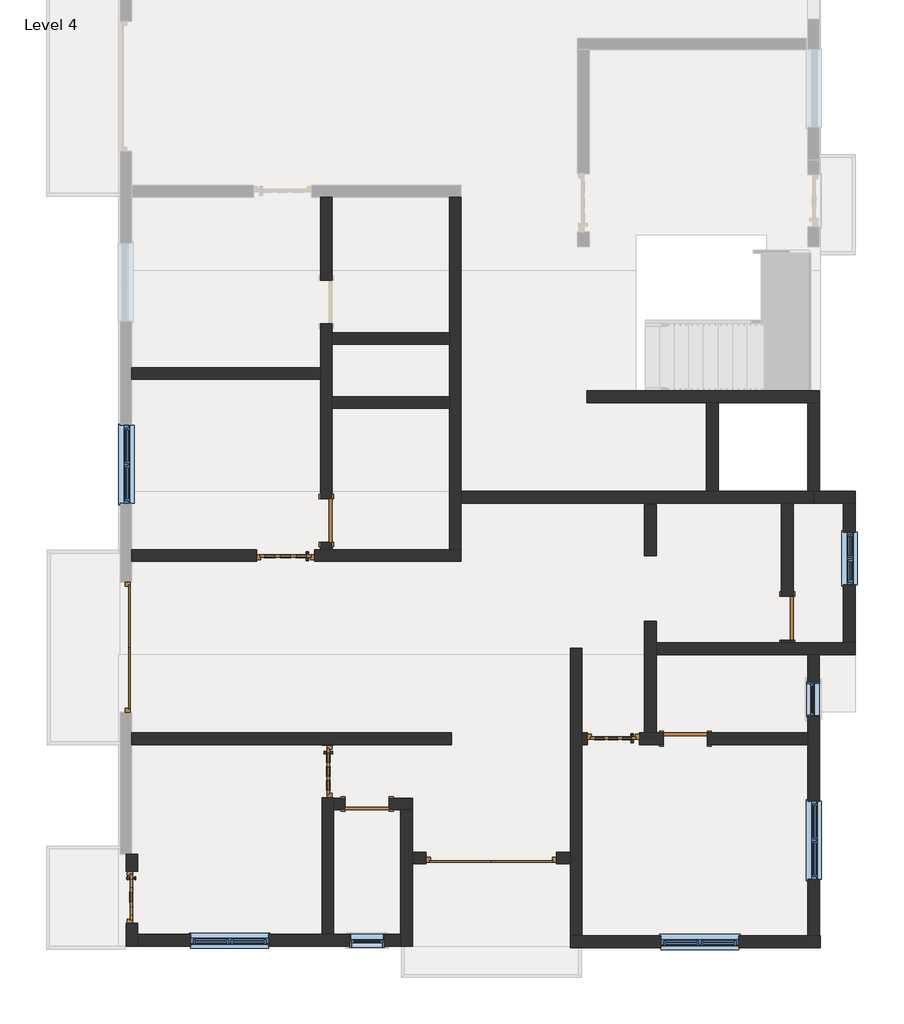
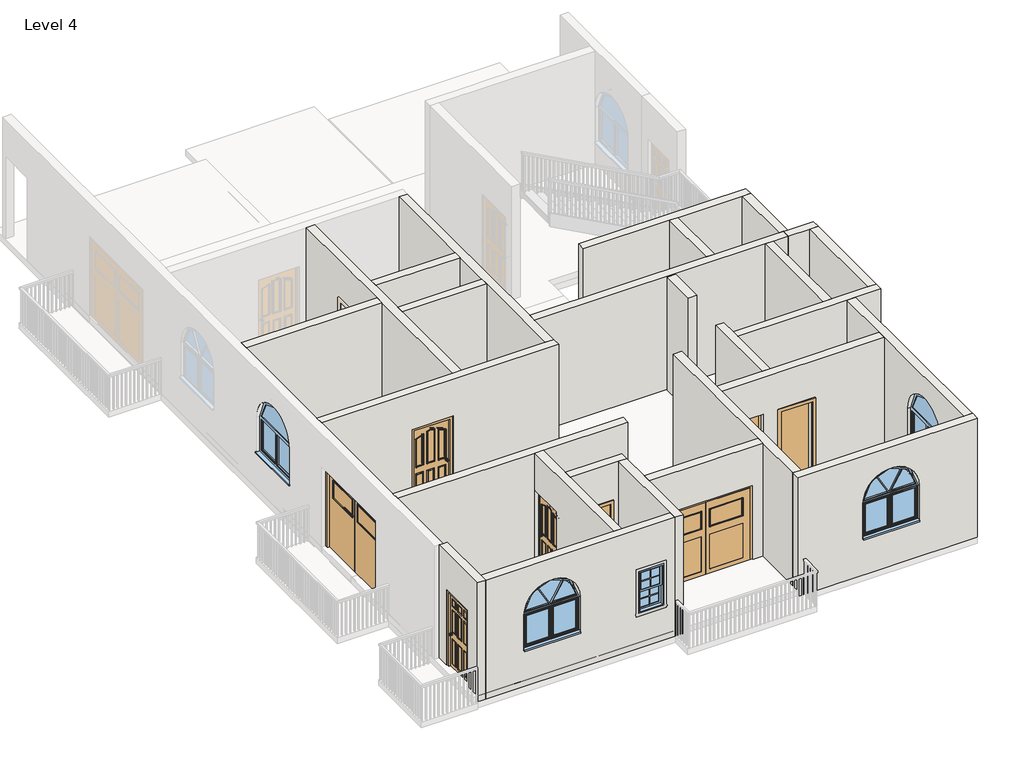
# One storey, part 1 of 7: 27 walls, 10 doors, 7 windows.
# Revit data of these elements (continued)
# Type "Single-Flush : 30\" x 80\"" (continued)
#   Construction Type Id = "MDOOR"
#   Assembly Code = "C1020"
#   Analytic Construction = "Metal"
#   Thickness = 0' - 2"
#   Heat Transfer Coefficient (U) = 0.651978 BTU/(h·ft²·°F)
#   Height = 6' - 8"
#   Trim Projection Ext = 0' - 1"
#   Trim Projection Int = 0' - 1"
#   Trim Width = 0' - 3"
#   Width = 2' - 6"
#   Define Thermal Properties by = 1
#   Define Thermal Properties by = 1
#   Door Material = Door - Panel
#   Frame Material = Door - Frame
#   Visual Light Transmittance = 0
#   Solar Heat Gain Coefficient = 0
#   Function = (empty or 0)
#   Wall Closure = (empty or 0)
# Type "Generic - 9\" w"
#   Assembly Code = "B2010"
#   Layers, outside or top first: 0' - 8" no material (function 1)
# Type "Generic -4.5\" p"
#   Assembly Code = "B2010"
#   Layers, outside or top first: 0' - 8" no material (function 1)
# Type "Window-Double-Hung : 24\" x 42\""
#   Type Mark = "10"
#   Fire Rating = "0.5h"
#   Construction Type Id = "DG-DR"
#   Assembly Code = "B2020100"
#   Analytic Construction = "Double glazing - domestic"
#   Wall Thickness [instance default] = 0' - 6"
#   Window Inset [instance default] = 0' - 0"
#   Visual Light Transmittance = 0.81
#   Thermal Resistance (R) = 1.8146 (h·ft²·°F)/BTU
#   Solar Heat Gain Coefficient = 0.76
#   Muntin Width = 1' - 6"
#   Muntin Height = 1' - 5 1/8"
#   Interior Wall Closure [instance default] = 0' - 1 1/2"
#   Rough Width = 2' - 0 1/2"
#   Rough Height = 3' - 6 1/2"
#   Frame Extension [instance default] = 0' - 1 1/4"
#   Exterior Wall Closure [instance default] = 0' - 0 1/2"
#   Extension Jamb [instance default] = 0' - 1 1/2"
#   Heat Transfer Coefficient (U) = 0.5511 BTU/(h·ft²·°F)
#   Height = 3' - 6"
#   Width = 2' - 0"
#   Define Thermal Properties by = 1
#   Top Muntin Visibility = yes
#   Indicator Visibility [instance default] = yes
#   Extension Jamb Visibility [instance default] = yes
#   Interior Trim Visibility [instance default] = yes
#   Exterior Trim Visibility [instance default] = yes
#   Define Thermal Properties by = 1
#   Bottom Muntin Visibility = yes
#   Muntin Pattern = Muntin Pattern_2x2 : Muntin Pattern_2x2
#   Interior Trim Material = Wood - Stained
#   Interior Trim = Trim-Window-Interior-Flat : Picture Frame
#   Exterior Trim Material = Clad - White
#   Exterior Trim = Trim-Window-Exterior-Flat : with Sill
#   Glass Panel Material = Glass
#   Exterior Frame Material = Clad - White
#   Interior Frame Material = Wood - Stained
#   Wall Closure = (empty or 0)
# Type "Windows_Arched : 1360x910mm"
#   Type Mark = "20"
#   Operation = "UserDefined"
#   Construction Type Id = "GSP4R"
#   Manufacturer = "Revit"
#   Keynote = "L10"
#   Analytic Construction = "1/8 in Pilkington single glazing"
#   Wrap Layers (Ext) from Ext = 0' - 4.03543"
#   Wrap Layers (Int) from Ext = 0' - 6.98819"
#   Window Board Projection = 0' - 0.98425"
#   Window Board Extension = 0' - 0.98425"
#   Visual Light Transmittance = 0.9
#   Solar Heat Gain Coefficient = 0.78
#   Rough Width = 4' - 5.54331"
#   Rough Height = 2' - 11.82677"
#   Height = 2' - 11.82677"
#   Width = 4' - 5.54331"
#   Heat Transfer Coefficient (U) = 0.6496 BTU/(h·ft²·°F)
#   Glazing Thickness = 0' - 0.94488"
#   FrameOffset - External = 0' - 1.9685"
#   Frame Depth = 0' - 2.67717"
#   Default Head Height = 6' - 11.07087"
#   Cill Depth = 0' - 3.44488"
#   Cavity Closer Width = 0' - 1.9685"
#   Cavity Closer Offset from Ext = 0' - 4.03543"
#   Cavity Closer Depth = 0' - 3.34646"
#   Vis - Cavity Closers = yes
#   Define Thermal Properties by = 1
#   Material Trim = Window Frame
#   Material Glass = Glass
#   Material Frame = Window Frame
#   Wall Closure = (empty or 0)
# Type "Windows_Dbl_w-Glazing_Bars : 910x910mm"
#   Type Mark = "33"
#   Operation = "DoublePanelVertical"
#   Construction Type Id = "GSP4R"
#   Manufacturer = "Revit"
#   Keynote = "L10"
#   Analytic Construction = "1/8 in Pilkington single glazing"
#   Wrap Layers (Ext) from Ext = 0' - 4.03543"
#   Wrap Layers (Int) from Ext = 0' - 6.98819"
#   Window Board Projection = 0' - 0.98425"
#   Window Board Extension = 0' - 0.98425"
#   Visual Light Transmittance = 0.9
#   Solar Heat Gain Coefficient = 0.78
#   Rough Width = 2' - 11.82677"
#   Rough Height = 2' - 11.82677"
#   Height = 2' - 11.82677"
#   Width = 2' - 11.82677"
#   Heat Transfer Coefficient (U) = 0.6496 BTU/(h·ft²·°F)
#   Glazing Thickness = 0' - 0.94488"
#   Glazing Bar Thickness = 0' - 0.7874"
#   FrameOffset - External = 0' - 1.9685"
#   Frame Depth = 0' - 2.55906"
#   Default Head Height = 6' - 10.67717"
#   Cill Depth = 0' - 3.44488"
#   Cavity Closer Width = 0' - 1.9685"
#   Cavity Closer Offset from Ext = 0' - 4.03543"
#   Cavity Closer Depth = 0' - 3.34646"
#   Vis - Glazing Bars = yes
#   Vis - Cavity Closers = yes
#   Define Thermal Properties by = 1
#   Material Trim = Window Frame
#   Material Glazing Bars = Window Frame
#   Material Glass = Glass
#   Material Frame = Window Frame
#   Wall Closure = (empty or 0)
# Element 1 (IfcDoor, "Doors_ExtSgl_5 : 910x2110mm")
#   Phase Created = New Construction
#   Materials on its faces: "Door - Panel", "Door - Handle", "Door - Frame/Mullion", "Door - Glazing"
# Element 2 (IfcDoor, "Doors_ExtSgl_6 : 1010x2110mm")
#   Phase Created = New Construction
#   Materials on its faces: "Door - Panel", "Door - Handle", "Door - Frame/Mullion", "Door - Glazing"
# Elements 3, 4 (IfcDoor, "Doors_ExtSgl_6 : 910x2110mm")
#   Phase Created = New Construction
#   Materials on its faces: "Door - Panel", "Door - Handle", "Door - Frame/Mullion", "Door - Glazing"
# Element 5 (IfcDoor, "Doors_Garage_Timber_Side_Hung_Glazing : 2270x2050mm")
#   Phase Created = New Construction
#   Materials on its faces: "Door - Panel", "Door - Frame/Mullion", "Door - Glazing"
# Element 6 (IfcDoor, "Doors_Garage_Timber_Side_Hung_Glazing : 2270x2200mm")
#   Phase Created = New Construction
#   Materials on its faces: "Door - Panel", "Door - Frame/Mullion", "Door - Glazing"
# Elements 7, 8, 9, 10 (IfcDoor, "Single-Flush : 30\" x 80\"")
#   Phase Created = New Construction
#   Materials on its faces: "Door - Frame", "Door - Panel"
# Element 11 (IfcWall, "Generic - 9\" w")
#   Top Offset = 0' - 0"
#   Base Offset = 0' - 0"
#   wall height = 10' - 0"
#   Phase Created = New Construction
#   Base Constraint = Level 4
#   Top Constraint = Level 5
#   Materials on its faces: "Default Wall", "Door - Frame", "Earth"
# Elements 12, 13 (IfcWall, "Generic - 9\" w")
#   Top Offset = 0' - 0"
#   Base Offset = 0' - 0"
#   wall height = 10' - 0"
#   Phase Created = New Construction
#   Base Constraint = Level 4
#   Top Constraint = Level 5
#   Materials on its faces: "Default Wall"
# Element 14 (IfcWall, "Generic - 9\" w")
#   Top Offset = 0' - 0"
#   Base Offset = 0' - 0"
#   wall height = 10' - 0"
#   Phase Created = New Construction
#   Base Constraint = Level 4
#   Top Constraint = Level 5
#   Materials on its faces: "Default Wall", "Door - Frame/Mullion", "Earth"
# Element 15 (IfcWall, "Generic - 9\" w")
#   Top Offset = 0' - 0"
#   Base Offset = 0' - 0"
#   wall height = 10' - 0"
#   Phase Created = New Construction
#   Base Constraint = Level 4
#   Top Constraint = Level 5
#   Materials on its faces: "Default Wall", "Concrete, Lightweight", "Wood - Stained"
# Element 16 (IfcWall, "Generic - 9\" w")
#   Top Offset = 0' - 0"
#   Base Offset = 0' - 0"
#   wall height = 10' - 0"
#   Phase Created = New Construction
#   Base Constraint = Level 4
#   Top Constraint = Level 5
#   Materials on its faces: "Default Wall", "Wood - Stained"
# Element 17 (IfcWall, "Generic - 9\" w")
#   Top Offset = 0' - 0"
#   Base Offset = 0' - 0"
#   wall height = 10' - 0"
#   Phase Created = New Construction
#   Base Constraint = Level 4
#   Top Constraint = Level 5
#   Materials on its faces: "Default Wall", "Earth"
# Element 18 (IfcWall, "Generic - 9\" w")
#   Top Offset = 0' - 0"
#   Base Offset = 0' - 0"
#   wall height = 10' - 0"
#   Phase Created = New Construction
#   Base Constraint = Level 4
#   Top Constraint = Level 5
#   Materials on its faces: "Default Wall", "Concrete, Lightweight"
# Element 19 (IfcWall, "Generic - 9\" w")
#   Top Offset = 0' - 0"
#   Base Offset = 0' - 0"
#   wall height = 10' - 0"
#   Phase Created = New Construction
#   Base Constraint = Level 4
#   Top Constraint = Level 5
#   Materials on its faces: "Default Wall", "Concrete, Lightweight", "Default Mass Interior Wall"
# Elements 20, 21, 22, 23, 24, 25, 26, 27, 28, 31, 32, 33, 36, 37 (IfcWall, "Generic -4.5\" p")
#   Top Offset = 0' - 0"
#   Base Offset = 0' - 0"
#   wall height = 10' - 0"
#   Phase Created = New Construction
#   Base Constraint = Level 4
#   Top Constraint = Level 5
#   Materials on its faces: "Default Wall"
# Element 29 (IfcWall, "Generic -4.5\" p")
#   Top Offset = 0' - 0"
#   Base Offset = 0' - 0"
#   wall height = 10' - 0"
#   Phase Created = New Construction
#   Base Constraint = Level 4
#   Top Constraint = Level 5
#   Materials on its faces: "Default Wall", "Concrete, Lightweight"
# Element 30 (IfcWall, "Generic -4.5\" p")
#   Top Offset = 0' - 0"
#   Base Offset = 0' - 0"
#   wall height = 10' - 0"
#   Phase Created = New Construction
#   Base Constraint = Level 4
#   Top Constraint = Level 5
#   Materials on its faces: "Default Wall", "Door - Frame/Mullion"
# Elements 34, 35 (IfcWall, "Generic -4.5\" p")
#   Top Offset = 0' - 0"
#   Base Offset = 0' - 0"
#   wall height = 10' - 0"
#   Phase Created = New Construction
#   Base Constraint = Level 4
#   Top Constraint = Level 5
#   Materials on its faces: "Default Wall", "Earth"
# Element 38 (IfcWindow, "Window-Double-Hung : 24\" x 42\"")
#   Mark = "49"
#   Window Inset = 0' - 0"
#   Interior Wall Closure = 0' - 1 1/2"
#   Frame Extension = 0' - 1 1/4"
#   Exterior Wall Closure = 0' - 0 1/2"
#   Interior Trim Visibility = yes
#   Indicator Visibility = yes
#   Exterior Trim Visibility = yes
#   Phase Created = New Construction
#   Materials on its faces: "Wood - Stained", "Glass", "Clad - White"
# Element 39 (IfcWindow, "Window-Double-Hung : 24\" x 42\"")
#   Mark = "90"
#   Window Inset = 0' - 0"
#   Interior Wall Closure = 0' - 1 1/2"
#   Frame Extension = 0' - 1 1/4"
#   Exterior Wall Closure = 0' - 0 1/2"
#   Interior Trim Visibility = yes
#   Indicator Visibility = yes
#   Exterior Trim Visibility = yes
#   Phase Created = New Construction
#   Materials on its faces: "Wood - Stained", "Glass", "Clad - White"
# Element 40 (IfcWindow, "Windows_Arched : 1360x910mm")
#   Mark = "45"
#   Phase Created = New Construction
#   Materials on its faces: "Window Frame", "Glass"
# Element 41 (IfcWindow, "Windows_Arched : 1360x910mm")
#   Mark = "46"
#   Phase Created = New Construction
#   Materials on its faces: "Window Frame", "Glass"
# Element 42 (IfcWindow, "Windows_Arched : 1360x910mm")
#   Mark = "47"
#   Phase Created = New Construction
#   Materials on its faces: "Window Frame", "Glass"
# Element 43 (IfcWindow, "Windows_Arched : 1360x910mm")
#   Mark = "85"
#   Phase Created = New Construction
#   Materials on its faces: "Window Frame", "Glass"
# Element 44 (IfcWindow, "Windows_Dbl_w-Glazing_Bars : 910x910mm")
#   Mark = "50"
#   Phase Created = New Construction
#   Materials on its faces: "Window Frame", "Glass"
# Materials
#   "Door - Glazing": colour RGB 0 0 255, transparency 0.75
#   "Door - Panel": class "Wood", colour RGB 210 159 95, transparency 0, Cost = 0
#   "Door - Frame/Mullion": class "Wood", colour RGB 212 179 113, transparency 0
#   "Door - Handle": colour RGB 0 0 0, transparency 0
#   "Door - Frame": colour RGB 118 70 51, transparency 0, Cost = 0
#   "Wood - Stained": class "Wood", colour RGB 224 178 126, transparency 0, Cost = 0
#   "Clad - White": class "Wood", colour RGB 242 242 238, transparency 0, Cost = 0
#   "Glass": class "Glass", colour RGB 0 128 192, transparency 0.75, Description = "Soda Lime Glass", Cost = 0
#   "Window Frame": colour RGB 249 249 249, transparency 0
#   "Default Wall": colour RGB 128 128 128, transparency 0, Cost = 0
#   "Earth": class "Generic", colour RGB 97 75 62, transparency 0, Description = "Soil", Cost = 0
#   "Concrete, Lightweight": class "Concrete", colour RGB 142 141 140, transparency 0, Description = "Lightweight concrete", Cost = 0
#   "Default Mass Interior Wall": class "Generic", colour RGB 195 229 126, transparency 0, Cost = 0
